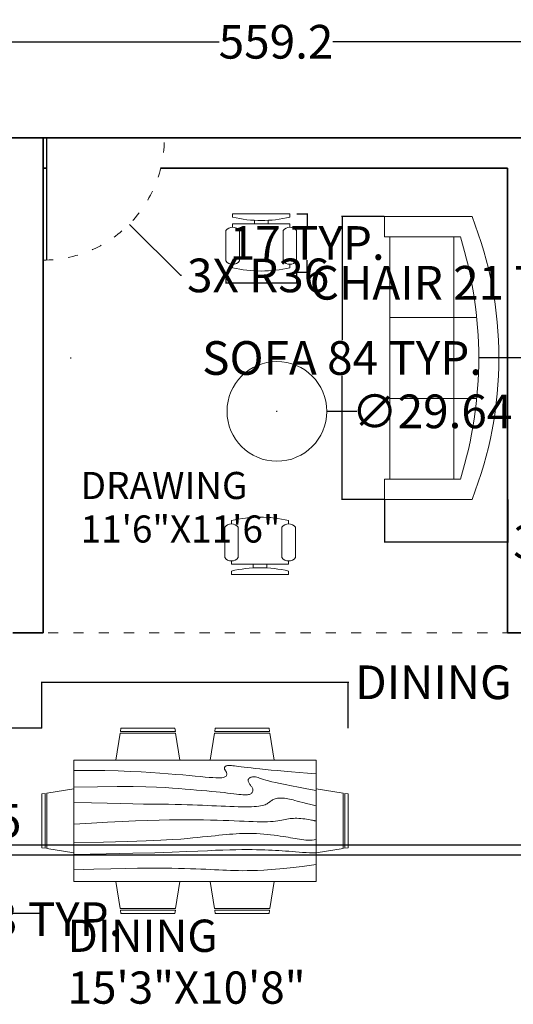
# Model space of a CAD drawing. Units: inches. Extents: x 37 to 687, y -399 to 163.
# Tile 3 of 4: x 286 to 432, y -129 to 163. Entities that reach past the tile are written whole.
import ezdxf

# ---------------------------------------------------------------- set-up
doc = ezdxf.new("R2010")
doc.units = ezdxf.units.IN
doc.header["$MEASUREMENT"] = 0
doc.linetypes.add('ACAD_ISO03W100', pattern=[30, 12, -18])
for name, color, linetype, lineweight in [('A-ANNO-DIMS', 2, 'Continuous', 18), ('A-AREA-IDEN', 7, 'Continuous', 18), ('A-DOOR', 4, 'Continuous', 25), ('A-DOOR-SWNG', 4, 'ACAD_ISO03W100', 13), ('A-FURN', 8, 'Continuous', 18), ('A-WALL', 7, 'Continuous', 35), ('A-WALL-OVHD', 7, 'ACAD_ISO03W100', 18)]:
    doc.layers.add(name, color=color, linetype=linetype, lineweight=lineweight)
doc.styles.get("Standard").update_dxf_attribs({"font": 'arial.ttf'})
doc.dimstyles.get("Standard").update_dxf_attribs({"dimtxt": 10, "dimasz": 0.18, "dimexe": 0.18, "dimexo": 0.0625, "dimgap": 0.09, "dimtad": 0, "dimtih": 1, "dimtoh": 1, "dimdec": 0, "dimzin": 0, "dimdsep": 46, "dimlunit": 3, "dimtxsty": 'Standard', "dimcen": 0.09, "dimadec": 0, "dimazin": 0, "dimtfac": 1, "dimtdec": 0, "dimtofl": 0, "dimtmove": 0, "dimatfit": 3, "dimfxl": 1, "dimtolj": 1, "dimtzin": 0, "dimarcsym": 0})

# ---------------------------------------------------------------- blocks, each defined once
blk = doc.blocks.new('Sofa - Roundback 7 ft.')
for p, q in [((-12.00002, -32.4421), (-12.00003, -6.5971)), ((11.99997, -32.4421), (11.99998, -6.5971)), ((-36.000027, -34), (-36.000027, -11.4696)), ((35.99998, -34), (35.99998, -11.4696)), ((-35.999844, -13.3819), (35.9998, -13.3819)), ((-36.000027, -32.4421), (35.99998, -32.4421))]:
    blk.add_line(p, q)
for points in [[(-36.000027, -34), (-42.000027, -34), (-42.000027, -8)], [(41.99998, -8), (41.99998, -34), (35.99998, -34)]]:
    blk.add_lwpolyline(points)
for centre, radius, start, end in [((0, -114.25), 114.25, 68.43141, 111.5686), ((-0.00001, -127.1968), 121.1968, 72.72033, 107.2797)]:
    blk.add_arc(centre, radius, start, end)
blk = doc.blocks.new('Chair - Desk')
for p, q in [((-8.5, 0), (-8.5, -1)), ((-8.5, 0), (8.5, 0)), ((8.5, 0), (8.5, -1)), ((-2, -3), (-2, -1.9355)), ((2, -1.9576), (2, -3)), ((-10.5, -5), (-10.5, -14)), ((-8.5, -3), (-8.5, -4)), ((-8.5, -3), (8.5, -3)), ((-6.5, -14), (-6.5, -5)), ((6.5, -5), (6.5, -14)), ((8.5, -3), (8.5, -4)), ((10.5, -14), (10.5, -5)), ((-8.5, -15), (-8.5, -16)), ((8.5, -15), (8.5, -16))]:
    blk.add_line(p, q)
for centre, radius, start, end in [((0, 34.625), 36.625, 256.5803, 283.4197), ((-8.5, -6.5), 2.5, 36.8699, 143.1301), ((8.5, -6.5), 2.5, 36.8699, 143.1301), ((-8.5, -12.5), 2.5, 216.8699, 323.1301), ((8.5, -12.5), 2.5, 216.8699, 323.1301), ((0, 19.625), 36.625, 256.5803, 283.4197)]:
    blk.add_arc(centre, radius, start, end)
blk = doc.blocks.new('Dining Set - 36 x 72 in.')
for p, q in [((-22, 27.5), (-22.1562, 26.50042)), ((-5.8416, 26.5), (-22.1534, 26.5)), ((-22, 27.5), (-6, 27.5)), ((-5.8437, 26.49966), (-6, 27.5)), ((6, 27.5), (5.8438, 26.50042)), ((22.1584, 26.5), (5.8466, 26.5)), ((6, 27.5), (22, 27.5)), ((22.1563, 26.49966), (22, 27.5)), ((-22.2343, 26.00059), (-23.4847, 17.99762)), ((-22.2304, 26), (-5.7608, 26)), ((-4.5152, 17.99762), (-5.7655, 25.99926)), ((5.7657, 26.00059), (4.5153, 17.99762)), ((5.7696, 26), (22.2392, 26)), ((23.4848, 17.99762), (22.2345, 25.99926)), ((36, 18), (-36, 18)), ((-36, 18), (-36, -18)), ((36, -18), (36, 18)), ((-44.0006, 8.23428), (-35.9976, 9.48474)), ((44.0006, 8.23428), (35.9976, 9.48474)), ((-45.5, 8), (-44.5004, 8.15617)), ((-45.5, 8), (-45.5, -8)), ((-44.5, -8.15843), (-44.5, 8.15338)), ((-44, 8.23041), (-44, -8.23915)), ((44, 8.23041), (44, -8.23915)), ((44.5, -8.15843), (44.5, 8.15338)), ((45.5, 8), (44.5005, 8.15617)), ((45.5, 8), (45.5, -8)), ((-44.4997, -8.15631), (-45.5, -8)), ((-35.9976, -9.48476), (-43.9993, -8.2345)), ((35.9976, -9.48476), (43.9993, -8.2345)), ((44.4997, -8.15631), (45.5, -8)), ((-36, -18), (36, -18)), ((-22.2343, -26.0006), (-23.4847, -17.99762)), ((-4.5152, -17.99762), (-5.7655, -25.99928)), ((5.7657, -26.0006), (4.5153, -17.99762)), ((23.4848, -17.99762), (22.2345, -25.99928)), ((-22.2304, -26), (-5.7608, -26)), ((5.7696, -26), (22.2392, -26)), ((-22, -27.5), (-22.1562, -26.50044)), ((-5.8416, -26.5), (-22.1534, -26.5)), ((-22, -27.5), (-6, -27.5)), ((-5.8437, -26.49967), (-6, -27.5)), ((6, -27.5), (5.8438, -26.50044)), ((22.1584, -26.5), (5.8466, -26.5)), ((6, -27.5), (22, -27.5)), ((22.1563, -26.49967), (22, -27.5))]:
    blk.add_line(p, q)
for points in [[(-36, 15), (-31.1772, 14.97754), (-26.8079, 14.91406), (-22.8538, 14.81543), (-19.276, 14.6875), (-16.0362, 14.53613), (-13.0957, 14.36718), (-10.4159, 14.18652), (-7.9583, 14), (-5.6904, 13.81315), (-3.6035, 13.63021), (-1.6954, 13.45508), (0.0365, 13.29166), (1.5945, 13.14388), (2.9811, 13.01562), (4.1988, 12.9108), (5.25, 12.83333), (6.1393, 12.78613), (6.8802, 12.76823), (7.4883, 12.77767), (7.9792, 12.8125), (8.3685, 12.87077), (8.6719, 12.95052), (8.9049, 13.0498), (9.0833, 13.16666), (9.2205, 13.29899), (9.3216, 13.44401), (9.3895, 13.59879), (9.4271, 13.76041), (9.4373, 13.92594), (9.4232, 14.09245), (9.3875, 14.257), (9.3333, 14.41666), (9.2638, 14.56917), (9.1836, 14.71484), (9.0975, 14.85465), (9.0104, 14.98958), (8.9272, 15.1206), (8.8529, 15.2487), (8.7922, 15.37483), (8.75, 15.5), (8.7305, 15.62467), (8.7344, 15.74739), (8.7617, 15.86621), (8.8125, 15.97916), (8.8867, 16.08431), (8.9844, 16.17968), (9.1055, 16.26334), (9.25, 16.33333), (9.4189, 16.38802), (9.6172, 16.42708), (9.8506, 16.45052), (10.125, 16.45833), (10.4463, 16.45052), (10.8203, 16.42708), (11.2529, 16.38802), (11.75, 16.33333), (12.3184, 16.26318), (12.9694, 16.17838), (13.7151, 16.07991), (14.5677, 15.96875), (15.5395, 15.84586), (16.6426, 15.71224), (17.8893, 15.56884), (19.2917, 15.41666), (20.859, 15.25667), (22.5879, 15.08984), (24.4721, 14.91715), (26.5052, 14.73958), (28.6809, 14.5581), (30.9929, 14.3737), (33.4347, 14.18733), (36, 14)], [(-36, 10), (-28.9766, 10.14274), (-23.1725, 10.20442), (-18.4241, 10.19775), (-14.5677, 10.13541), (-11.4399, 10.03011), (-8.877, 9.89453), (-6.7154, 9.74137), (-4.7917, 9.58333), (-2.9698, 9.43082), (-1.2246, 9.28515), (0.4415, 9.14534), (2.026, 9.01041), (3.5266, 8.87939), (4.9408, 8.7513), (6.266, 8.62516), (7.5, 8.5), (8.6411, 8.37549), (9.6914, 8.2539), (10.6538, 8.13818), (11.5312, 8.03125), (12.3267, 7.93603), (13.043, 7.85547), (13.6831, 7.79248), (14.25, 7.75), (14.7471, 7.7303), (15.1797, 7.73307), (15.5537, 7.75732), (15.875, 7.80208), (16.1494, 7.86637), (16.3828, 7.94922), (16.5811, 8.04964), (16.75, 8.16666), (16.8944, 8.29915), (17.0143, 8.44531), (17.1089, 8.60319), (17.1771, 8.77083), (17.218, 8.94629), (17.2305, 9.1276), (17.2137, 9.31282), (17.1667, 9.5), (17.0895, 9.6875), (16.987, 9.875), (16.8649, 10.0625), (16.7292, 10.25), (16.5856, 10.4375), (16.4401, 10.625), (16.2985, 10.8125), (16.1667, 11), (16.05, 11.18733), (15.9518, 11.3737), (15.8752, 11.5581), (15.8229, 11.73958), (15.798, 11.91715), (15.8034, 12.08984), (15.842, 12.25667), (15.9167, 12.41666), (16.0295, 12.56836), (16.1784, 12.70833), (16.3605, 12.83268), (16.5729, 12.9375), (16.8127, 13.01888), (17.0768, 13.07291), (17.3625, 13.0957), (17.6667, 13.08333), (17.9894, 13.03312), (18.3418, 12.94726), (18.7382, 12.82918), (19.1927, 12.68229), (19.7195, 12.51001), (20.3327, 12.31575), (21.0465, 12.10294), (21.875, 11.875), (22.8357, 11.63354), (23.959, 11.37304), (25.2786, 11.08618), (26.8282, 10.76562), (28.6414, 10.40405), (30.752, 9.99414), (33.1936, 9.52856), (36, 9)], [(-36, 5.5), (-30.7157, 5.3348), (-26.069, 5.20963), (-21.9946, 5.11767), (-18.4271, 5.05208), (-15.3009, 5.00602), (-12.5508, 4.97265), (-10.1112, 4.94515), (-7.9167, 4.91666), (-5.909, 4.88167), (-4.0586, 4.83984), (-2.3429, 4.79215), (-0.7396, 4.73958), (0.7739, 4.6831), (2.22, 4.6237), (3.6213, 4.56233), (5, 4.5), (6.373, 4.43782), (7.7344, 4.3776), (9.0723, 4.32129), (10.375, 4.27083), (11.6309, 4.22819), (12.8281, 4.19531), (13.9551, 4.17415), (15, 4.16666), (15.954, 4.17448), (16.819, 4.19791), (17.6001, 4.23698), (18.3021, 4.29166), (18.9299, 4.36198), (19.4883, 4.44791), (19.9823, 4.54948), (20.4167, 4.66666), (20.7969, 4.79899), (21.1302, 4.94401), (21.4245, 5.09879), (21.6875, 5.26041), (21.9271, 5.42594), (22.1511, 5.59245), (22.3672, 5.757), (22.5834, 5.91666), (22.8065, 6.06868), (23.0404, 6.21093), (23.2879, 6.34147), (23.5521, 6.45833), (23.8358, 6.55957), (24.142, 6.64323), (24.4735, 6.70735), (24.8334, 6.75), (25.2235, 6.76969), (25.642, 6.76692), (26.0858, 6.74267), (26.5521, 6.69791), (27.0379, 6.63362), (27.5404, 6.55078), (28.0565, 6.45036), (28.5834, 6.33333), (29.1242, 6.19987), (29.7071, 6.04687), (30.3661, 5.87044), (31.1354, 5.66666), (32.0493, 5.43164), (33.142, 5.16146), (34.4475, 4.85221), (36, 4.5)], [(-36, -1), (-30.7915, -0.6591), (-26.0195, -0.38216), (-21.6519, -0.16284), (-17.6563, 0.00521), (-14.0005, 0.12833), (-10.6523, 0.21289), (-7.5796, 0.26522), (-4.75, 0.29166), (-2.134, 0.29793), (0.2878, 0.28711), (2.5317, 0.26163), (4.6146, 0.22396), (6.5529, 0.17651), (8.3633, 0.12174), (10.0623, 0.06209), (11.6667, 0), (13.1899, -0.06201), (14.6341, -0.1211), (15.9982, -0.17432), (17.2813, -0.21875), (18.4823, -0.25147), (19.6003, -0.26953), (20.6343, -0.27002), (21.5834, -0.25), (22.4481, -0.20768), (23.2357, -0.14584), (23.9549, -0.06836), (24.6146, 0.02083), (25.2235, 0.11784), (25.7904, 0.21875), (26.3241, 0.31966), (26.8334, 0.41666), (27.3265, 0.50618), (27.8099, 0.58593), (28.2894, 0.65397), (28.7709, 0.70833), (29.2601, 0.74707), (29.763, 0.76823), (30.2855, 0.76985), (30.8334, 0.75), (31.4088, 0.70784), (31.9994, 0.64713), (32.589, 0.57275), (33.1615, 0.48958), (33.7008, 0.4025), (34.1908, 0.3164), (34.6153, 0.23616), (34.9584, 0.16666), (35.2099, 0.11165), (35.3848, 0.07031), (35.504, 0.04069), (35.5886, 0.02083), (35.6594, 0.00879), (35.7377, 0.0026), (35.8442, 0.00032), (36, 0)], [(-36, -6.5), (-27.1843, -6.31267), (-20.084, -6.1263), (-14.469, -5.9419), (-10.1094, -5.76042), (-6.7752, -5.58285), (-4.2363, -5.41016), (-2.2629, -5.24333), (-0.625, -5.08334), (0.8708, -4.93099), (2.2715, -4.78646), (3.5872, -4.64974), (4.8281, -4.52084), (6.0046, -4.39974), (7.127, -4.28646), (8.2053, -4.18099), (9.25, -4.08334), (10.2705, -3.99382), (11.2734, -3.91407), (12.2647, -3.84603), (13.25, -3.79167), (14.2354, -3.75293), (15.2266, -3.73177), (16.2295, -3.73015), (17.25, -3.75), (18.2912, -3.79248), (19.3451, -3.85547), (20.4009, -3.93604), (21.4479, -4.03125), (22.4754, -4.13819), (23.4727, -4.25391), (24.4289, -4.37549), (25.3334, -4.5), (26.1785, -4.62492), (26.9694, -4.74935), (27.7145, -4.87281), (28.4219, -4.99479), (29.1, -5.11483), (29.7572, -5.23242), (30.4016, -5.34709), (31.0417, -5.45834), (31.6837, -5.56437), (32.3262, -5.65821), (32.9658, -5.73153), (33.599, -5.77604), (34.2224, -5.78345), (34.8327, -5.74545), (35.4264, -5.65373), (36, -5.5)], [(-36, -10), (-26.4022, -9.81299), (-18.4675, -9.62891), (-11.9839, -9.45069), (-6.7396, -9.28125), (-2.5226, -9.12354), (0.8789, -8.98047), (3.6769, -8.85498), (6.0833, -8.75), (8.2767, -8.66765), (10.3021, -8.60677), (12.1712, -8.56543), (13.8958, -8.54167), (15.4876, -8.53353), (16.9583, -8.53907), (18.3197, -8.55632), (19.5834, -8.58334), (20.7616, -8.61841), (21.8685, -8.66081), (22.9188, -8.71004), (23.9271, -8.76563), (24.9081, -8.82707), (25.8763, -8.89388), (26.8465, -8.96558), (27.8334, -9.04167), (28.8474, -9.12118), (29.8828, -9.20117), (30.93, -9.27824), (31.9792, -9.34896), (33.0205, -9.40991), (34.0443, -9.45768), (35.0407, -9.48885), (36, -9.5)], [(-36, -14.5), (-30.0881, -14.33513), (-25.0332, -14.21224), (-20.7312, -14.12647), (-17.0781, -14.07292), (-13.97, -14.04671), (-11.3027, -14.04297), (-8.9724, -14.05681), (-6.875, -14.08334), (-4.9224, -14.11833), (-3.0905, -14.16016), (-1.3709, -14.20785), (0.2448, -14.26042), (1.7647, -14.3169), (3.1973, -14.3763), (4.5507, -14.43767), (5.8333, -14.5), (7.0554, -14.5621), (8.235, -14.62175), (9.3922, -14.67652), (10.5469, -14.72396), (11.7192, -14.76164), (12.929, -14.78711), (14.1965, -14.79794), (15.5417, -14.79167), (16.9933, -14.76424), (18.6152, -14.70508), (20.4804, -14.60197), (22.6615, -14.44271), (25.2312, -14.21509), (28.2624, -13.9069), (31.8277, -13.50594), (36, -13)]]:
    blk.add_lwpolyline(points)
blk = doc.blocks.new('*D11')
at = {"layer": 'A-ANNO-DIMS', "color": 0, "lineweight": -2, "ltscale": 0.25, "transparency": 16777216}
for p, q in [((347, 88.33), (347, 85.06)), ((368, 88.33), (368, 85.06)), ((347.18, 85.24), (367.82, 85.24)), ((368, 85.24), (368.18, 85.24))]:
    blk.add_line(p, q, dxfattribs=at)
at = {"layer": 'A-ANNO-DIMS', "color": 0, "ltscale": 0.25, "transparency": 16777216}
for points in [[(347.18, 85.27), (347.18, 85.21), (347, 85.24)], [(367.82, 85.27), (367.82, 85.21), (368, 85.24)]]:
    blk.add_solid(points, dxfattribs=at)
at = {"layer": 'Defpoints', "color": 0, "ltscale": 0.25, "transparency": 16777216}
for p in [(347, 88.39), (368, 88.39), (368, 85.24)]:
    blk.add_point(p, dxfattribs=at)
at = {"layer": 'A-ANNO-DIMS', "color": 0, "ltscale": 0.25, "transparency": 16777216, "insert": (416.22, 85.24), "char_height": 10, "attachment_point": 5}
blk.add_mtext('\\A1;CHAIR 21 TYP.', dxfattribs=at)
blk = doc.blocks.new('*D12')
at = {"layer": 'A-ANNO-DIMS', "color": 0, "lineweight": -2, "ltscale": 0.25, "transparency": 16777216}
for p, q in [((368.06, 105.73), (371.33, 105.73)), ((371.15, 105.55), (371.15, 102.17)), ((371.15, 88.57), (371.15, 91.95)), ((368.06, 88.39), (371.33, 88.39))]:
    blk.add_line(p, q, dxfattribs=at)
at = {"layer": 'A-ANNO-DIMS', "color": 0, "ltscale": 0.25, "transparency": 16777216}
for points in [[(371.12, 105.55), (371.18, 105.55), (371.15, 105.73)], [(371.12, 88.57), (371.18, 88.57), (371.15, 88.39)]]:
    blk.add_solid(points, dxfattribs=at)
at = {"layer": 'Defpoints', "color": 0, "ltscale": 0.25, "transparency": 16777216}
for p in [(368, 105.73), (371.15, 105.73), (368, 88.39)]:
    blk.add_point(p, dxfattribs=at)
at = {"layer": 'A-ANNO-DIMS', "color": 0, "ltscale": 0.25, "transparency": 16777216, "insert": (371.15, 97.06), "char_height": 10, "attachment_point": 5}
blk.add_mtext('\\A1;17 TYP.', dxfattribs=at)
blk = doc.blocks.new('*D17')
at = {"layer": 'A-ANNO-DIMS', "color": 0, "lineweight": -2, "ltscale": 0.25, "transparency": 16777216}
for p, q in [((209.64, -108.64), (209.64, -103.57)), ((209.82, -103.75), (242.51, -103.75)), ((242.69, -108.64), (242.69, -103.57)), ((242.69, -103.75), (242.87, -103.75))]:
    blk.add_line(p, q, dxfattribs=at)
at = {"layer": 'A-ANNO-DIMS', "color": 0, "ltscale": 0.25, "transparency": 16777216}
for points in [[(209.82, -103.72), (209.82, -103.78), (209.64, -103.75)], [(242.51, -103.72), (242.51, -103.78), (242.69, -103.75)]]:
    blk.add_solid(points, dxfattribs=at)
at = {"layer": 'Defpoints', "color": 0, "ltscale": 0.25, "transparency": 16777216}
for p in [(242.69, -103.75), (209.64, -108.71), (242.69, -108.71)]:
    blk.add_point(p, dxfattribs=at)
at = {"layer": 'A-ANNO-DIMS', "color": 0, "ltscale": 0.25, "transparency": 16777216, "insert": (281.08, -103.75), "char_height": 10, "attachment_point": 5}
blk.add_mtext('\\A1;WC 33 TYP.', dxfattribs=at)
blk = doc.blocks.new('*D19')
at = {"layer": 'A-ANNO-DIMS', "color": 0, "lineweight": -2, "ltscale": 0.25, "transparency": 16777216}
for p, q in [((394.06, 104.9), (381.34, 104.9)), ((381.52, 104.72), (381.52, 68.16)), ((381.52, 21.08), (381.52, 57.64)), ((394.06, 20.9), (381.34, 20.9))]:
    blk.add_line(p, q, dxfattribs=at)
at = {"layer": 'A-ANNO-DIMS', "color": 0, "ltscale": 0.25, "transparency": 16777216}
for points in [[(381.49, 104.72), (381.55, 104.72), (381.52, 104.9)], [(381.49, 21.08), (381.55, 21.08), (381.52, 20.9)]]:
    blk.add_solid(points, dxfattribs=at)
at = {"layer": 'Defpoints', "color": 0, "ltscale": 0.25, "transparency": 16777216}
for p in [(394.12, 104.9), (381.52, 20.9), (394.12, 20.9)]:
    blk.add_point(p, dxfattribs=at)
at = {"layer": 'A-ANNO-DIMS', "color": 0, "ltscale": 0.25, "transparency": 16777216, "insert": (381.52, 62.9), "char_height": 10, "attachment_point": 5}
blk.add_mtext('\\A1;SOFA 84 TYP.', dxfattribs=at)
blk = doc.blocks.new('*D20')
at = {"layer": 'A-ANNO-DIMS', "color": 0, "lineweight": -2, "ltscale": 0.25, "transparency": 16777216}
for p, q in [((394.12, 20.84), (394.12, 8.12)), ((430.79, 20.84), (430.79, 8.12)), ((394.3, 8.3), (430.61, 8.3)), ((430.79, 8.3), (430.97, 8.3))]:
    blk.add_line(p, q, dxfattribs=at)
at = {"layer": 'A-ANNO-DIMS', "color": 0, "ltscale": 0.25, "transparency": 16777216}
for points in [[(394.3, 8.33), (394.3, 8.27), (394.12, 8.3)], [(430.61, 8.33), (430.61, 8.27), (430.79, 8.3)]]:
    blk.add_solid(points, dxfattribs=at)
at = {"layer": 'Defpoints', "color": 0, "ltscale": 0.25, "transparency": 16777216}
for p in [(394.12, 20.9), (430.79, 20.9), (430.79, 8.3)]:
    blk.add_point(p, dxfattribs=at)
at = {"layer": 'A-ANNO-DIMS', "color": 0, "ltscale": 0.25, "transparency": 16777216, "insert": (455.39, 8.3), "char_height": 10, "attachment_point": 5}
blk.add_mtext('\\A1;37 TYP.', dxfattribs=at)
blk = doc.blocks.new('*D21')
at = {"layer": 'A-ANNO-DIMS', "color": 0, "lineweight": -2, "ltscale": 0.25, "transparency": 16777216}
for p, q in [((292.31, -47.01), (292.31, -33.24)), ((292.49, -33.42), (383.13, -33.42)), ((383.31, -47.01), (383.31, -33.24)), ((383.31, -33.42), (383.49, -33.42))]:
    blk.add_line(p, q, dxfattribs=at)
at = {"layer": 'A-ANNO-DIMS', "color": 0, "ltscale": 0.25, "transparency": 16777216}
for points in [[(292.49, -33.39), (292.49, -33.45), (292.31, -33.42)], [(383.13, -33.39), (383.13, -33.45), (383.31, -33.42)]]:
    blk.add_solid(points, dxfattribs=at)
at = {"layer": 'Defpoints', "color": 0, "ltscale": 0.25, "transparency": 16777216}
for p in [(383.31, -33.42), (292.31, -47.07), (383.31, -47.07)]:
    blk.add_point(p, dxfattribs=at)
at = {"layer": 'A-ANNO-DIMS', "color": 0, "ltscale": 0.25, "transparency": 16777216, "insert": (431.44, -33.42), "char_height": 10, "attachment_point": 5}
blk.add_mtext('\\A1;DINING SET 91', dxfattribs=at)
blk = doc.blocks.new('*D22')
at = {"layer": 'A-ANNO-DIMS', "color": 0, "lineweight": -2, "ltscale": 0.25, "transparency": 16777216}
for p, q in [((292.25, -47.07), (278.48, -47.07)), ((278.66, -47.25), (278.66, -69.4)), ((278.66, -101.89), (278.66, -79.75)), ((292.25, -102.07), (278.48, -102.07))]:
    blk.add_line(p, q, dxfattribs=at)
at = {"layer": 'A-ANNO-DIMS', "color": 0, "ltscale": 0.25, "transparency": 16777216}
for points in [[(278.63, -47.25), (278.69, -47.25), (278.66, -47.07)], [(278.63, -101.89), (278.69, -101.89), (278.66, -102.07)]]:
    blk.add_solid(points, dxfattribs=at)
at = {"layer": 'Defpoints', "color": 0, "ltscale": 0.25, "transparency": 16777216}
for p in [(278.66, -47.07), (292.31, -47.07), (292.31, -102.07)]:
    blk.add_point(p, dxfattribs=at)
at = {"layer": 'A-ANNO-DIMS', "color": 0, "ltscale": 0.25, "transparency": 16777216, "insert": (278.66, -74.57), "char_height": 10, "attachment_point": 5}
blk.add_mtext('\\A1;55', dxfattribs=at)
blk = doc.blocks.new('*D27')
at = {"layer": 'A-ANNO-DIMS', "color": 0, "lineweight": -2, "ltscale": 0.25, "transparency": 16777216}
for p, q in [((82.29, -12.62), (82.29, 157)), ((82.47, 156.82), (344.98, 156.82)), ((641.3, 156.82), (378.8, 156.82)), ((641.48, 53.47), (641.48, 157))]:
    blk.add_line(p, q, dxfattribs=at)
at = {"layer": 'A-ANNO-DIMS', "color": 0, "ltscale": 0.25, "transparency": 16777216}
for points in [[(82.47, 156.85), (82.47, 156.79), (82.29, 156.82)], [(641.3, 156.85), (641.3, 156.79), (641.48, 156.82)]]:
    blk.add_solid(points, dxfattribs=at)
at = {"layer": 'Defpoints', "color": 0, "ltscale": 0.25, "transparency": 16777216}
for p in [(641.48, 156.82), (641.48, 53.4), (82.29, -12.68)]:
    blk.add_point(p, dxfattribs=at)
at = {"layer": 'A-ANNO-DIMS', "color": 0, "ltscale": 0.25, "transparency": 16777216, "insert": (361.89, 156.82), "char_height": 10, "attachment_point": 5}
blk.add_mtext('\\A1;559.2', dxfattribs=at)
blk = doc.blocks.new('*D44')
at = {"layer": 'A-ANNO-DIMS', "color": 0, "lineweight": -2, "ltscale": 0.25, "transparency": 16777216}
for p, q in [((242.75, -81.68), (670.18, -81.68)), ((670, -81.68), (670, -81.5)), ((670, -81.5), (670.18, -81.5)), ((670, -84.5), (670, -81.86)), ((242.75, -84.68), (670.18, -84.68))]:
    blk.add_line(p, q, dxfattribs=at)
at = {"layer": 'A-ANNO-DIMS', "color": 0, "ltscale": 0.25, "transparency": 16777216}
for points in [[(669.97, -81.86), (670.03, -81.86), (670, -81.68)], [(669.97, -84.5), (670.03, -84.5), (670, -84.68)]]:
    blk.add_solid(points, dxfattribs=at)
at = {"layer": 'Defpoints', "color": 0, "ltscale": 0.25, "transparency": 16777216}
for p in [(242.69, -81.68), (670, -81.68), (242.69, -84.68)]:
    blk.add_point(p, dxfattribs=at)
at = {"layer": 'A-ANNO-DIMS', "color": 0, "ltscale": 0.25, "transparency": 16777216, "insert": (673.54, -81.5), "char_height": 10, "attachment_point": 5}
blk.add_mtext('\\A1;3', dxfattribs=at)
blk = doc.blocks.new('*D45')
at = {"layer": 'A-ANNO-DIMS', "color": 0, "lineweight": -2, "ltscale": 0.25, "transparency": 16777216}
for p, q in [((362.05, 47.06), (362.23, 47.06)), ((362.14, 46.97), (362.14, 47.15)), ((385.85, 47.05), (377.14, 47.05))]:
    blk.add_line(p, q, dxfattribs=at)
at = {"layer": 'A-ANNO-DIMS', "color": 0, "ltscale": 0.25, "transparency": 16777216}
blk.add_solid([(377.14, 47.08), (377.14, 47.02), (376.96, 47.05)], dxfattribs=at)
at = {"layer": 'Defpoints', "color": 0, "ltscale": 0.25, "transparency": 16777216}
for p in [(347.32, 47.06), (376.96, 47.05)]:
    blk.add_point(p, dxfattribs=at)
at = {"layer": 'A-ANNO-DIMS', "color": 0, "ltscale": 0.25, "transparency": 16777216, "insert": (408.24, 47.05), "char_height": 10, "attachment_point": 5}
blk.add_mtext('\\A1;∅29.64', dxfattribs=at)
blk = doc.blocks.new('*D48')
at = {"layer": 'A-ANNO-DIMS', "color": 0, "lineweight": -2, "ltscale": 0.25, "transparency": 16777216}
for p, q in [((292.6, 127.97), (292.78, 127.97)), ((292.69, 127.88), (292.69, 128.06)), ((333.61, 87.43), (318.39, 102.51)), ((333.79, 87.43), (333.61, 87.43))]:
    blk.add_line(p, q, dxfattribs=at)
at = {"layer": 'A-ANNO-DIMS', "color": 0, "ltscale": 0.25, "transparency": 16777216}
blk.add_solid([(318.41, 102.53), (318.37, 102.49), (318.26, 102.63)], dxfattribs=at)
at = {"layer": 'Defpoints', "color": 0, "ltscale": 0.25, "transparency": 16777216}
for p in [(292.69, 127.97), (318.26, 102.63)]:
    blk.add_point(p, dxfattribs=at)
at = {"layer": 'A-ANNO-DIMS', "color": 0, "ltscale": 0.25, "transparency": 16777216, "insert": (356.57, 87.43), "char_height": 10, "attachment_point": 5}
blk.add_mtext('\\A1;3X R36', dxfattribs=at)
blk = doc.blocks.new('*D54')
at = {"layer": 'A-ANNO-DIMS', "color": 0, "lineweight": -2, "ltscale": 0.25, "transparency": 16777216}
for p, q in [((300.83, 62.9), (301.01, 62.9)), ((300.92, 62.81), (300.92, 62.99)), ((494.84, 62.9), (422.3, 62.9))]:
    blk.add_line(p, q, dxfattribs=at)
at = {"layer": 'A-ANNO-DIMS', "color": 0, "ltscale": 0.25, "transparency": 16777216}
blk.add_solid([(422.3, 62.93), (422.3, 62.87), (422.12, 62.9)], dxfattribs=at)
at = {"layer": 'Defpoints', "color": 0, "ltscale": 0.25, "transparency": 16777216}
for p in [(300.92, 62.9), (422.12, 62.9)]:
    blk.add_point(p, dxfattribs=at)
at = {"layer": 'A-ANNO-DIMS', "color": 0, "ltscale": 0.25, "transparency": 16777216, "insert": (527.36, 62.9), "char_height": 10, "attachment_point": 5}
blk.add_mtext('\\A1;2X R121.2', dxfattribs=at)

msp = doc.modelspace()

# ---------------------------------------------------------------- linework, layer by layer
at = {"layer": 'A-DOOR', "ltscale": 0.25}
for p, q in [((292.6852, 128.3154), (292.6852, 91.9677)), ((292.6852, 128.3154), (328.6852, 128.3154)), ((293.6852, 128.3154), (293.6852, 91.9677))]:
    msp.add_line(p, q, dxfattribs=at)
at = {"layer": 'A-DOOR-SWNG', "ltscale": 0.25}
msp.add_arc((292.6852, 127.9694), 36.0017, 270, 0.550698, dxfattribs=at)
at = {"layer": 'A-FURN', "ltscale": 0.25}
msp.add_circle((362.1415, 47.0552), 14.8205, dxfattribs=at)
at = {"layer": 'A-WALL'}
for p, q in [((137.6852, 128.3154), (595.6852, 128.3154)), ((292.6852, 128.3154), (292.6852, -12.6846)), ((292.6852, 128.3154), (430.6852, 128.3154)), ((292.6852, 119.3154), (293.6852, 119.3154)), ((327.6312, 119.3154), (430.6852, 119.3154)), ((430.6852, 119.3154), (430.6852, -18.6846)), ((292.6852, -18.6846), (292.6852, -12.6846))]:
    msp.add_line(p, q, dxfattribs=at)
at = {"layer": 'A-WALL', "ltscale": 0.25}
for p, q in [((292.6852, -18.6846), (283.6852, -18.6846)), ((439.6852, -18.6846), (430.6852, -18.6846))]:
    msp.add_line(p, q, dxfattribs=at)
at = {"layer": 'A-WALL-OVHD', "ltscale": 0.25}
msp.add_line((439.6852, -18.6846), (283.6852, -18.6846), dxfattribs=at)

# ---------------------------------------------------------------- block references
at = {"layer": 'A-FURN', "ltscale": 0.25}
for name, p in [('Chair - Desk', (357.5001, 105.727)), ('Dining Set - 36 x 72 in.', (337.8108, -74.5722))]:
    msp.add_blockref(name, p, dxfattribs=at)
for name, p, rotation in [('Sofa - Roundback 7 ft.', (428.1189, 62.8991), 270), ('Chair - Desk', (357.1278, -1.3818), 180)]:
    msp.add_blockref(name, p, dxfattribs=dict(at, rotation=rotation))

# ---------------------------------------------------------------- texts
at = {"layer": 'A-AREA-IDEN', "ltscale": 0.25}
for s, height, p in [('DRAWING', 8.04732, (303.8328, 21.0107)), ('11\'6"X11\'6"', 8.04732, (303.8328, 8.0834)), ('DINING', 9.58603, (299.9548, -113.4879)), ('15\'3"X10\'8"', 9.58603, (299.9548, -128.887))]:
    msp.add_text(s, height=height, dxfattribs=at).set_placement(p)

# ---------------------------------------------------------------- dimensions: what is measured, and where the dimension line sits
at = {"layer": 'A-ANNO-DIMS', "ltscale": 0.25}
dim = msp.add_linear_dim(base=(641.4841, 156.8154), p1=(82.2949, -12.6846), p2=(641.4841, 53.4042), dimstyle='Standard', override={"dimdec": 1, "dimlfac": 1, "dimrnd": 0, "dimzin": 0, "dimdsep": 46, "dimlunit": 2}, dxfattribs=at)
dim.commit()
dim.dimension.update_dxf_attribs({"geometry": '*D27', "text_midpoint": (361.8895, 156.8154)})
for center, mpoint, text, override, picture, middle in [((292.6852, 127.9694), (318.2641, 102.6349), '3X <>', {"dimdec": 0, "dimlfac": 1, "dimrnd": 0, "dimzin": 0, "dimdsep": 46, "dimlunit": 2}, '*D48', (356.5657, 87.4342)), ((300.9221, 62.8991), (422.1189, 62.899), '2X <>', {"dimdec": 1, "dimlfac": 1, "dimrnd": 0, "dimzin": 0, "dimdsep": 46, "dimlunit": 2}, '*D54', (494.837, 62.8989))]:
    dim = msp.add_radius_dim(center=center, mpoint=mpoint, text=text, dimstyle='Standard', override=override, dxfattribs=at)
    dim.commit()
    dim.dimension.update_dxf_attribs({"geometry": picture, "text_midpoint": middle, "dimtype": 164})
for base, p1, p2, angle, text, picture, middle in [((371.1501, 105.727), (368.0001, 88.3936), (368.0001, 105.727), 90, '<> TYP.', '*D12', (371.1501, 97.0603)), ((381.5189, 20.8991), (394.1189, 104.8991), (394.1189, 20.8991), 270, 'SOFA <> TYP.', '*D19', (381.5189, 62.8991)), ((242.6852, -103.7503), (209.6389, -108.7072), (242.6852, -108.7072), 0, 'WC <> TYP.', '*D17', (281.0759, -103.7503))]:
    dim = msp.add_linear_dim(base=base, p1=p1, p2=p2, angle=angle, text=text, dimstyle='Standard', override={"dimdec": 0, "dimlfac": 1, "dimrnd": 0, "dimzin": 0, "dimdsep": 46, "dimlunit": 2}, dxfattribs=at)
    dim.commit()
    dim.dimension.update_dxf_attribs({"geometry": picture, "text_midpoint": middle})
for base, p1, p2, text, picture, middle in [((368.0001, 85.2436), (347.0001, 88.3936), (368.0001, 88.3936), 'CHAIR <> TYP.', '*D11', (416.2237, 85.2436)), ((430.7856, 8.2991), (394.1189, 20.8991), (430.7856, 20.8991), '<> TYP.', '*D20', (455.3905, 8.2991)), ((383.3108, -33.4222), (292.3108, -47.0722), (383.3108, -47.0722), 'DINING SET <>', '*D21', (431.4423, -33.4222))]:
    dim = msp.add_linear_dim(base=base, p1=p1, p2=p2, text=text, dimstyle='Standard', override={"dimdec": 0, "dimlfac": 1, "dimrnd": 0, "dimzin": 0, "dimdsep": 46, "dimlunit": 2}, dxfattribs=at)
    dim.commit()
    dim.dimension.update_dxf_attribs({"geometry": picture, "text_midpoint": middle})
dim = msp.add_diameter_dim_2p(p1=(347.321, 47.0555), p2=(376.962, 47.055), dimstyle='Standard', override={"dimdec": 2, "dimlfac": 1, "dimrnd": 0, "dimzin": 0, "dimdsep": 46, "dimlunit": 2}, dxfattribs=at)
dim.commit()
dim.dimension.update_dxf_attribs({"geometry": '*D45', "text_midpoint": (385.8543, 47.0549), "dimtype": 163})
for base, p1, p2, picture, middle in [((278.6608, -47.0722), (292.3108, -102.0722), (292.3108, -47.0722), '*D22', (278.6608, -74.5722)), ((669.9983, -81.6846), (242.6852, -84.6846), (242.6852, -81.6846), '*D44', (673.5425, -81.5046))]:
    dim = msp.add_linear_dim(base=base, p1=p1, p2=p2, angle=90, dimstyle='Standard', override={"dimdec": 0, "dimlfac": 1, "dimrnd": 0, "dimzin": 0, "dimdsep": 46, "dimlunit": 2}, dxfattribs=at)
    dim.commit()
    dim.dimension.update_dxf_attribs({"geometry": picture, "text_midpoint": middle})

doc.saveas('drawing.dxf')
